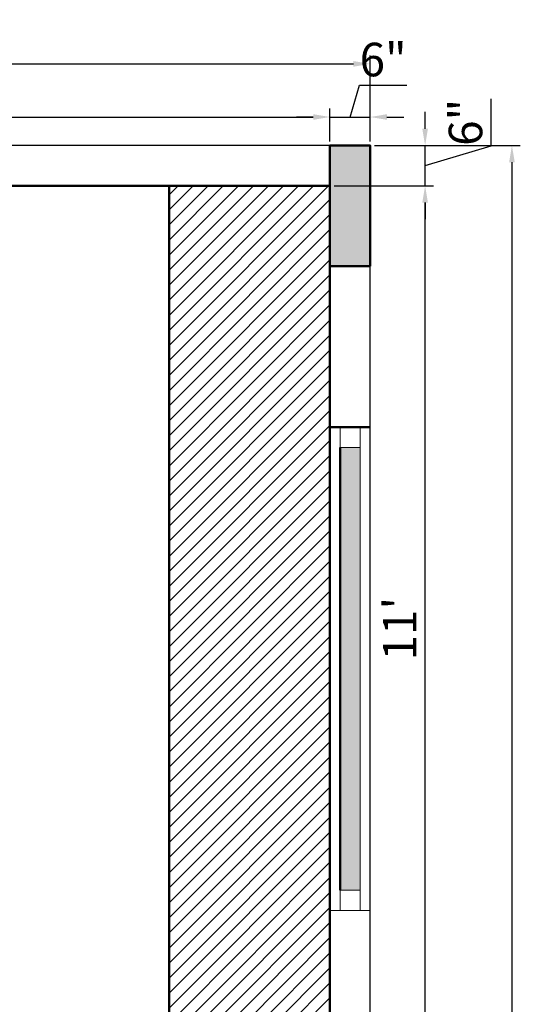
# Model space of a CAD drawing. Units: inches. Extents: x 3064 to 19385, y 846 to 15425.
# Tile 34 of 108: x 5054 to 5129, y 1264 to 1411. Entities that reach past the tile are written whole.
import ezdxf

# ---------------------------------------------------------------- set-up
doc = ezdxf.new("R2010")
doc.units = ezdxf.units.IN
for name, color, linetype, lineweight in [('A-ANNO-DIMS', 2, 'Continuous', 18), ('A-COLS', 1, 'Continuous', 35), ('A-FURN-PATT', 252, 'Continuous', 13), ('A-GLAZ', 4, 'Continuous', 18), ('A-WALL', 7, 'Continuous', 50), ('C-PROP', 6, 'Continuous', 25)]:
    doc.layers.add(name, color=color, linetype=linetype, lineweight=lineweight)
doc.styles.get("Standard").update_dxf_attribs({"font": 'arial.ttf'})
doc.dimstyles.new('ISO-25', dxfattribs={"dimtxt": 9, "dimasz": 2.5, "dimexe": 1.25, "dimexo": 0.625, "dimtad": 1, "dimdec": 1, "dimlunit": 3, "dimtxsty": 'Standard', "dimcen": 2.5, "dimadec": 0, "dimazin": 0, "dimtfac": 1, "dimtdec": 1, "dimtmove": 0, "dimatfit": 3, "dimfxl": 1, "dimarcsym": 0})

# ---------------------------------------------------------------- blocks, each defined once
blk = doc.blocks.new('*D46')
at = {"layer": 'A-ANNO-DIMS', "color": 0, "lineweight": -2, "transparency": 16777216}
for p, q in [((4905.48, 1392.72), (4905.48, 1397.6)), ((5100.48, 1392.72), (5100.48, 1397.6)), ((4907.98, 1396.35), (5097.98, 1396.35))]:
    blk.add_line(p, q, dxfattribs=at)
at = {"layer": 'A-ANNO-DIMS', "color": 0, "transparency": 16777216}
for points in [[(4907.98, 1396.77), (4907.98, 1395.93), (4905.48, 1396.35)], [(5097.98, 1396.77), (5097.98, 1395.93), (5100.48, 1396.35)]]:
    blk.add_solid(points, dxfattribs=at)
at = {"layer": 'Defpoints', "color": 0, "transparency": 16777216}
for p in [(5100.48, 1396.35), (4905.48, 1392.1), (5100.48, 1392.1)]:
    blk.add_point(p, dxfattribs=at)
at = {"layer": 'A-ANNO-DIMS', "color": 0, "transparency": 16777216, "insert": (5002.98, 1399.53), "char_height": 5, "attachment_point": 5}
blk.add_mtext('16\'-3"', dxfattribs=at)
blk = doc.blocks.new('*D47')
at = {"layer": 'A-ANNO-DIMS', "color": 0, "lineweight": -2, "transparency": 16777216}
for p, q in [((5103.48, 1396.35), (5104.9, 1401.09)), ((5104.9, 1401.09), (5111.92, 1401.09)), ((5100.48, 1392.72), (5100.48, 1397.6)), ((5106.48, 1392.72), (5106.48, 1397.6)), ((5097.98, 1396.35), (5095.48, 1396.35)), ((5100.48, 1396.35), (5106.48, 1396.35)), ((5100.48, 1396.35), (5106.48, 1396.35)), ((5108.98, 1396.35), (5111.48, 1396.35))]:
    blk.add_line(p, q, dxfattribs=at)
at = {"layer": 'A-ANNO-DIMS', "color": 0, "transparency": 16777216}
for points in [[(5097.98, 1396.77), (5097.98, 1395.93), (5100.48, 1396.35)], [(5108.98, 1396.77), (5108.98, 1395.93), (5106.48, 1396.35)]]:
    blk.add_solid(points, dxfattribs=at)
at = {"layer": 'Defpoints', "color": 0, "transparency": 16777216}
for p in [(5106.48, 1396.35), (5100.48, 1392.1), (5106.48, 1392.1)]:
    blk.add_point(p, dxfattribs=at)
at = {"layer": 'A-ANNO-DIMS', "color": 0, "transparency": 16777216, "insert": (5108.41, 1404.27), "char_height": 5, "attachment_point": 5}
blk.add_mtext('6"', dxfattribs=at)
blk = doc.blocks.new('*D64')
at = {"layer": 'A-ANNO-DIMS', "color": 0, "lineweight": -2, "transparency": 16777216}
for p, q in [((5101.1, 1386.1), (5115.92, 1386.1)), ((5114.67, 1256.6), (5114.67, 1383.6)), ((5107.1, 1254.1), (5115.92, 1254.1))]:
    blk.add_line(p, q, dxfattribs=at)
at = {"layer": 'A-ANNO-DIMS', "color": 0, "transparency": 16777216}
for points in [[(5114.25, 1383.6), (5115.09, 1383.6), (5114.67, 1386.1)], [(5114.25, 1256.6), (5115.09, 1256.6), (5114.67, 1254.1)]]:
    blk.add_solid(points, dxfattribs=at)
at = {"layer": 'Defpoints', "color": 0, "transparency": 16777216}
for p in [(5100.48, 1386.1), (5114.67, 1386.1), (5106.48, 1254.1)]:
    blk.add_point(p, dxfattribs=at)
at = {"layer": 'A-ANNO-DIMS', "color": 0, "transparency": 16777216, "insert": (5111.53, 1320.1), "char_height": 5, "attachment_point": 5, "rotation": 90}
blk.add_mtext("11'", dxfattribs=at)
blk = doc.blocks.new('*D65')
at = {"layer": 'A-ANNO-DIMS', "color": 0, "lineweight": -2, "transparency": 16777216}
for p, q in [((5124.52, 1392.05), (5124.52, 1399.07)), ((5114.67, 1394.6), (5114.67, 1397.1)), ((5107.1, 1392.1), (5115.92, 1392.1)), ((5114.67, 1386.1), (5114.67, 1392.1)), ((5114.67, 1386.1), (5114.67, 1392.1)), ((5114.67, 1389.1), (5124.52, 1392.05)), ((5101.1, 1386.1), (5115.92, 1386.1)), ((5114.67, 1383.6), (5114.67, 1381.1))]:
    blk.add_line(p, q, dxfattribs=at)
at = {"layer": 'A-ANNO-DIMS', "color": 0, "transparency": 16777216}
for points in [[(5114.25, 1394.6), (5115.09, 1394.6), (5114.67, 1392.1)], [(5114.25, 1383.6), (5115.09, 1383.6), (5114.67, 1386.1)]]:
    blk.add_solid(points, dxfattribs=at)
at = {"layer": 'Defpoints', "color": 0, "transparency": 16777216}
for p in [(5106.48, 1392.1), (5114.67, 1392.1), (5100.48, 1386.1)]:
    blk.add_point(p, dxfattribs=at)
at = {"layer": 'A-ANNO-DIMS', "color": 0, "transparency": 16777216, "insert": (5121.34, 1395.56), "char_height": 5, "attachment_point": 5, "rotation": 90}
blk.add_mtext('6"', dxfattribs=at)
blk = doc.blocks.new('*D66')
at = {"layer": 'A-ANNO-DIMS', "color": 0, "lineweight": -2, "transparency": 16777216}
for p, q in [((5107.1, 1392.1), (5128.87, 1392.1)), ((5127.62, 1389.6), (5127.62, 878.6)), ((5107.1, 876.1), (5128.87, 876.1))]:
    blk.add_line(p, q, dxfattribs=at)
at = {"layer": 'A-ANNO-DIMS', "color": 0, "transparency": 16777216}
for points in [[(5127.2, 1389.6), (5128.04, 1389.6), (5127.62, 1392.1)], [(5127.2, 878.6), (5128.04, 878.6), (5127.62, 876.1)]]:
    blk.add_solid(points, dxfattribs=at)
at = {"layer": 'Defpoints', "color": 0, "transparency": 16777216}
for p in [(5106.48, 1392.1), (5106.48, 876.1), (5127.62, 876.1)]:
    blk.add_point(p, dxfattribs=at)
at = {"layer": 'A-ANNO-DIMS', "color": 0, "transparency": 16777216, "insert": (5124.44, 1134.1), "char_height": 5, "attachment_point": 5, "rotation": 90}
blk.add_mtext("43'", dxfattribs=at)
blk = doc.blocks.new('*D67')
at = {"layer": 'A-ANNO-DIMS', "color": 0, "lineweight": -2, "transparency": 16777216}
for p, q in [((4764.48, 1392.72), (4764.48, 1405.52)), ((5106.48, 1392.72), (5106.48, 1405.52)), ((4766.98, 1404.27), (5103.98, 1404.27))]:
    blk.add_line(p, q, dxfattribs=at)
at = {"layer": 'A-ANNO-DIMS', "color": 0, "transparency": 16777216}
for points in [[(4766.98, 1404.69), (4766.98, 1403.85), (4764.48, 1404.27)], [(5103.98, 1404.69), (5103.98, 1403.85), (5106.48, 1404.27)]]:
    blk.add_solid(points, dxfattribs=at)
at = {"layer": 'Defpoints', "color": 0, "transparency": 16777216}
for p in [(5106.48, 1404.27), (4764.48, 1392.1), (5106.48, 1392.1)]:
    blk.add_point(p, dxfattribs=at)
at = {"layer": 'A-ANNO-DIMS', "color": 0, "transparency": 16777216, "insert": (4935.48, 1407.45), "char_height": 5, "attachment_point": 5}
blk.add_mtext('28\'-6"', dxfattribs=at)
blk = doc.blocks.new('WIN-1900')
blk.add_line((3, 0), (3, 66))
blk.add_lwpolyline([(3, 66), (0, 66), (0, 69), (3, 69)], close=True)

msp = doc.modelspace()

# ---------------------------------------------------------------- hatches: boundary and pattern name
at = {"layer": 'A-COLS'}
h = msp.add_hatch(color=256, dxfattribs=at)
h.dxf.hatch_style = 1
h.paths.add_polyline_path([(5106.48, 1374.1), (5106.48, 1392.1), (5100.48, 1392.1), (5100.48, 1374.1)])
at = {"layer": 'A-FURN-PATT'}
h = msp.add_hatch(dxfattribs=at)
h.set_pattern_fill('ANSI31', color=256, scale=0.5)
h.set_pattern_definition([(45, (-551.1915, -4.2436), (-1.122532, 1.122532), [])])
h.paths.add_polyline_path([(5076.48, 1254.1), (5100.48, 1254.1), (5100.48, 1386.1), (5076.48, 1386.1)])
at = {"layer": 'A-GLAZ'}
h = msp.add_hatch(color=256, dxfattribs=at)
h.dxf.hatch_style = 1
h.paths.add_polyline_path([(5101.98, 1281.1), (5104.98, 1281.1), (5104.98, 1347.1), (5101.98, 1347.1)])

# ---------------------------------------------------------------- linework, layer by layer
msp.add_line((5106.48, 1278.1), (5100.48, 1278.1), dxfattribs=at)
msp.add_lwpolyline([(5104.98, 1278.1), (5101.98, 1278.1), (5101.98, 1281.1), (5104.98, 1281.1)], close=True, dxfattribs=at)
at = {"layer": 'A-WALL'}
for p, q in [((5100.48, 1386.1), (4905.48, 1386.1)), ((5076.48, 1248.1), (5076.48, 1386.1)), ((5100.48, 1254.1), (5100.48, 1386.1)), ((5100.48, 1350.1), (5106.48, 1350.1)), ((5101.98, 1347.1), (5101.98, 1281.1))]:
    msp.add_line(p, q, dxfattribs=at)
msp.add_lwpolyline([(5106.48, 1374.1), (5106.48, 1392.1), (5100.48, 1392.1), (5100.48, 1374.1)], close=True, dxfattribs=at)
at = {"layer": 'C-PROP'}
for p, q in [((5106.48, 1392.1), (4764.48, 1392.1)), ((5106.48, 876.1), (5106.48, 1392.1))]:
    msp.add_line(p, q, dxfattribs=at)

# ---------------------------------------------------------------- block references
at = {"layer": 'A-GLAZ'}
msp.add_blockref('WIN-1900', (5101.98, 1281.1), dxfattribs=at)

# ---------------------------------------------------------------- dimensions: what is measured, and where the dimension line sits
at = {"layer": 'A-ANNO-DIMS'}
for base, p1, p2, override, picture, middle in [((5106.48, 1404.27), (4764.48, 1392.1), (5106.48, 1392.1), {"dimtxt": 5, "dimclrd": 0, "dimclre": 0, "dimclrt": 0}, '*D67', (4935.48, 1407.45)), ((5106.48, 1396.35), (5100.48, 1392.1), (5106.48, 1392.1), {"dimtxt": 5, "dimclrd": 0, "dimclre": 0, "dimclrt": 0, "dimtmove": 1}, '*D47', (5105.52, 1404.27)), ((5100.48, 1396.35), (4905.48, 1392.1), (5100.48, 1392.1), {"dimtxt": 5, "dimclrd": 0, "dimclre": 0, "dimclrt": 0, "dimtmove": 1}, '*D46', (5002.98, 1399.53))]:
    dim = msp.add_linear_dim(base=base, p1=p1, p2=p2, dimstyle='ISO-25', override=override, dxfattribs=at)
    dim.commit()
    dim.dimension.update_dxf_attribs({"geometry": picture, "text_midpoint": middle})
for base, p1, p2, override, picture, middle in [((5114.67, 1392.1), (5100.48, 1386.1), (5106.48, 1392.1), {"dimtxt": 5, "dimclrd": 0, "dimclre": 0, "dimclrt": 0, "dimtmove": 1}, '*D65', (5121.34, 1392.68)), ((5127.62, 876.1), (5106.48, 1392.1), (5106.48, 876.1), {"dimtxt": 5, "dimclrd": 0, "dimclre": 0, "dimclrt": 0}, '*D66', (5124.44, 1134.1)), ((5114.67, 1386.1), (5106.48, 1254.1), (5100.48, 1386.1), {"dimtxt": 5, "dimclrd": 0, "dimclre": 0, "dimclrt": 0, "dimtmove": 1}, '*D64', (5111.53, 1320.1))]:
    dim = msp.add_linear_dim(base=base, p1=p1, p2=p2, angle=90, dimstyle='ISO-25', override=override, dxfattribs=at)
    dim.commit()
    dim.dimension.update_dxf_attribs({"geometry": picture, "text_midpoint": middle})

doc.saveas('drawing.dxf')
